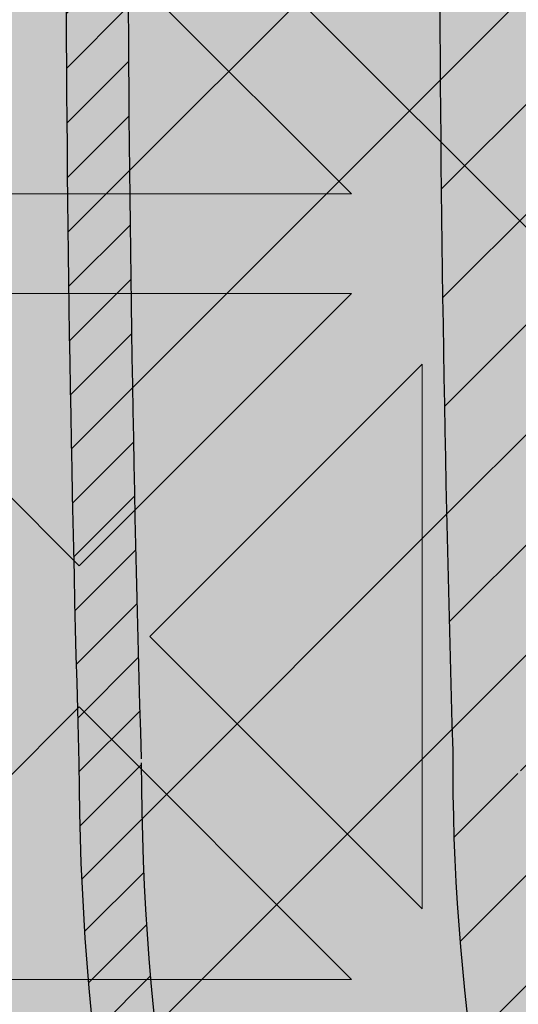
# Model space of a CAD drawing. Units: inches. Extents: x 844 to 2234, y 346 to 1084.
# Tile 11 of 93: x 1119.118 to 1120.394, y 691.183 to 693.702. Entities that reach past the tile are written whole.
import ezdxf

# ---------------------------------------------------------------- set-up
doc = ezdxf.new("R2010")
doc.units = ezdxf.units.IN
doc.header["$MEASUREMENT"] = 0
for name, color, linetype, lineweight in [('A-ANNO-DIMS', 2, 'Continuous', 18), ('furniture', 8, 'Continuous', 18), ('RA-AP-01$0$INT', 35, 'Continuous', 5)]:
    doc.layers.add(name, color=color, linetype=linetype, lineweight=lineweight)
doc.layers.add('RA-AP-01$0$FURN', color=3, linetype='Continuous')
doc.layers.add('RA-AP-01$0$WOOD', color=64, linetype='Continuous')
doc.styles.get("Standard").update_dxf_attribs({"font": 'arial.ttf'})
doc.dimstyles.get("Standard").update_dxf_attribs({"dimtxt": 6, "dimasz": 3, "dimexe": 0.18, "dimexo": 0.0625, "dimgap": 0.09, "dimtad": 0, "dimtih": 1, "dimtoh": 1, "dimdec": 1, "dimzin": 0, "dimdsep": 46, "dimlunit": 3, "dimtxsty": 'Standard', "dimblk": 'ARCHTICK', "dimcen": 0.09, "dimadec": 0, "dimazin": 0, "dimtfac": 1, "dimtdec": 1, "dimtofl": 0, "dimtmove": 0, "dimatfit": 3, "dimfxl": 1, "dimtolj": 1, "dimtzin": 0, "dimarcsym": 0})

# ---------------------------------------------------------------- blocks, each defined once
blk = doc.blocks.new('A$C18D01794')
at = {"layer": 'RA-AP-01$0$INT'}
h = blk.add_hatch(color=256, dxfattribs=at)
h.paths.add_polyline_path([(4.585917135068449, -6.356712009588271), (4.555206456959269, -6.35671200958746), (4.555206456959137, -6.387422687716308), (4.874495778835233, -6.706712009592356), (4.90520645695423, -6.676001331474049)])
h.paths.add_polyline_path([(5.255206456948813, -6.387422687716306), (5.255206456948682, -6.356712009605972), (5.224495778822613, -6.356712009605161), (4.905206456953498, -6.676001331474273), (4.935917135072151, -6.706712009592924)])
h.paths.add_polyline_path([(4.935917135072559, -6.706712009592068), (4.905206456953564, -6.737422687710376), (5.255206456951813, -7.087422687708613), (5.255206456951549, -7.026001331471008)])
h.paths.add_polyline_path([(4.555206456956399, -7.026001331471013), (4.555206456956134, -7.087422687708616), (4.905206456953821, -6.737422687710943), (4.874495778835166, -6.70671200959229)])
h = blk.add_hatch(color=256, dxfattribs=at)
h.paths.add_polyline_path([(4.585917135068448, -6.356712009588273), (4.614201406330596, -6.356712009589021), (4.668846067270487, -6.411356670531338), (4.723490728212344, -6.356712009591912), (4.771774999457151, -6.35671200959319), (4.826419660396886, -6.411356670535356), (4.862780050090322, -6.374996280843536), (4.844495778842715, -6.356712009595112), (4.862780050090411, -6.356712009595595), (4.905206456960182, -6.399138416468211), (4.947632863832445, -6.356712009597838), (4.965917135079675, -6.356712009598322), (4.947632863831759, -6.374996280845421), (4.983993253523576, -6.411356670538857), (5.038637914464627, -6.356712009600247), (5.08692218571208, -6.356712009601523), (5.141566846649976, -6.411356670541852), (5.196211507589851, -6.356712009604411), (5.224495778822615, -6.356712009605161), (4.905206456953975, -6.676001331473793)])
h.paths.add_polyline_path([(4.895206456956031, -6.637717060225675), (4.895206456958921, -6.528427738347902), (4.840561796018589, -6.583072399285802)], flags=16)
h.paths.add_polyline_path([(4.915206456955638, -6.637717060226121), (4.969851117895509, -6.583072399288678), (4.915206456957609, -6.528427738348344)], flags=16)
h.paths.add_polyline_path([(4.826419660395175, -6.568930263661755), (4.881064321335613, -6.514285602723745), (4.771774999456703, -6.514285602720857)], flags=16)
h.paths.add_polyline_path([(4.983993253519558, -6.568930263665262), (5.038637914460456, -6.514285602726792), (4.929348592581548, -6.514285602724816)], flags=16)
h.paths.add_polyline_path([(4.881064321336025, -6.494285602723742), (4.826419660397532, -6.439640941782821), (4.771774999457062, -6.494285602720859)], flags=16)
h.paths.add_polyline_path([(4.929348592582019, -6.494285602724817), (5.038637914460982, -6.494285602726792), (4.983993253522945, -6.439640941786327)], flags=16)
h.paths.add_polyline_path([(4.895206456960191, -6.480143467100443), (4.895206456962115, -6.407422687715913), (4.876922185715016, -6.389138416467584), (4.840561796021581, -6.425498806159401)], flags=16)
h.paths.add_polyline_path([(4.915206456958487, -6.480143467100889), (4.969851117899527, -6.425498806162279), (4.933490728206909, -6.389138416468043), (4.9152064569598, -6.40742268771434)], flags=16)
h.paths.add_polyline_path([(4.757632863832376, -6.480143467096812), (4.812277524772842, -6.425498806158772), (4.757632863834348, -6.370854145217844)], flags=16)
h.paths.add_polyline_path([(4.737632863832376, -6.480143467096286), (4.737632863834348, -6.370854145217375), (4.682988202893906, -6.425498806155385)], flags=16)
h.paths.add_polyline_path([(5.05278005008503, -6.480143467103376), (5.052780050087917, -6.370854145224413), (4.998135389146995, -6.425498806162908)], flags=16)
h.paths.add_polyline_path([(5.072780050085024, -6.480143467103744), (5.127424711025931, -6.42549880616527), (5.072780050087916, -6.370854145224832)], flags=16)
h.paths.add_polyline_path([(4.935917135072783, -6.706712009592292), (5.255206456948811, -6.387422687716309), (5.255206456948932, -6.415706958964177), (5.200561796010279, -6.470351619902839), (5.255206456949403, -6.524996280841948), (5.25520645694961, -6.5732805520894), (5.200561796009787, -6.627925213029239), (5.236922185702417, -6.664285602721864), (5.255206456949919, -6.646001331474357), (5.255206456949998, -6.664285602721898), (5.212780050078687, -6.706712009592262), (5.25520645695036, -6.749138416463932), (5.255206456950438, -6.767422687711313), (5.236922185702424, -6.749138416463297), (5.200561796009796, -6.785498806155928), (5.255206456950753, -6.840143467096874), (5.25520645695096, -6.888427738341682), (5.200561796010322, -6.943072399282328), (5.255206456951428, -6.997717060223427), (5.255206456951547, -7.026001331471006)])
h.paths.add_polyline_path([(5.042988202883395, -6.785498806155427), (5.097632863823085, -6.840143467095101), (5.097632863822622, -6.730854145216193)], flags=16)
h.paths.add_polyline_path([(5.028846067259663, -6.771356670531693), (5.083490728198774, -6.716712009592573), (4.974201406321001, -6.716712009593042)], flags=16)
h.paths.add_polyline_path([(5.117632863823087, -6.840143467095186), (5.172277524762331, -6.785498806155926), (5.11763286382262, -6.730854145216225)], flags=16)
h.paths.add_polyline_path([(5.08349072819877, -6.696712009593886), (5.028846067259652, -6.642067348654775), (4.974201406320998, -6.696712009593438)], flags=16)
h.paths.add_polyline_path([(5.131774999446817, -6.854285602718917), (5.186419660386065, -6.799640941779662), (5.241064321325782, -6.854285602719365)], flags=17)
h.paths.add_polyline_path([(5.131774999446228, -6.716712009592374), (5.186419660386065, -6.771356670532194), (5.222780050079488, -6.734996280838764), (5.204495778832781, -6.716712009592063)], flags=16)
h.paths.add_polyline_path([(5.097632863822613, -6.682569873970264), (5.097632863823061, -6.573280552091354), (5.042988202883383, -6.627925213031044)], flags=16)
h.paths.add_polyline_path([(5.131774999446899, -6.874285602718915), (5.241064321325809, -6.874285602719364), (5.186419660386591, -6.928930263658598)], flags=17)
h.paths.add_polyline_path([(5.131774999446226, -6.696712009594078), (5.204495778830767, -6.696712009594374), (5.22278005007868, -6.67842773834687), (5.186419660386049, -6.642067348654249)], flags=16)
h.paths.add_polyline_path([(5.11763286382262, -6.682569873970225), (5.17227752476232, -6.627925213030515), (5.117632863823064, -6.573280552091267)], flags=16)
h.paths.add_polyline_path([(5.186419660386069, -6.613783077405491), (5.241064321325754, -6.559138416465795), (5.131774999446791, -6.559138416466263)], flags=16)
h.paths.add_polyline_path([(5.131774999446872, -6.539138416466263), (5.24106432132578, -6.539138416465794), (5.186419660386554, -6.484493755526573)], flags=16)
h.paths.add_polyline_path([(5.255206456951811, -7.08742268770861), (5.255206456951895, -7.106712009588038), (4.555206456956052, -7.106712009588038), (4.555206456956136, -7.087422687708617), (4.905206456953973, -6.737422687710788)])
h.paths.add_polyline_path([(4.983993253513404, -6.8444937555241), (4.92934859257295, -6.899138416462108), (5.03863791445186, -6.899138416465014)], flags=16)
h.paths.add_polyline_path([(4.969851117889988, -6.83035161990006), (4.915206456952556, -6.775706958960171), (4.915206456949648, -6.884996280837944)], flags=16)
h.paths.add_polyline_path([(4.929348592572535, -6.919138416462105), (4.983993253511019, -6.973783077403037), (5.038637914451496, -6.919138416465012)], flags=16)
h.paths.add_polyline_path([(5.052780050074912, -6.93328055208906), (4.998135389134438, -6.987925213027088), (5.052780050072919, -7.042569873968025)], flags=16)
h.paths.add_polyline_path([(5.07278005007491, -6.933280552089588), (5.072780050072918, -7.042569873968497), (5.127424711013374, -6.987925213030498)], flags=16)
h.paths.add_polyline_path([(4.89520645695295, -6.775706958959721), (4.840561796013067, -6.830351619897157), (4.895206456950961, -6.884996280837494)], flags=16)
h.paths.add_polyline_path([(4.915206456948365, -6.933280552085403), (4.915206456946434, -7.006001331471951), (4.933490728192729, -7.024285602719066), (4.969851117886972, -6.987925213026453)], flags=16)
h.paths.add_polyline_path([(4.881064321327021, -6.899138416461022), (4.82641966038902, -6.84449375552057), (4.771774999448108, -6.899138416459029)], flags=16)
h.paths.add_polyline_path([(4.895206456950073, -6.933280552084951), (4.840561796009022, -6.987925213023558), (4.876922185700835, -7.024285602716997), (4.895206456948749, -7.006001331469487)], flags=16)
h.paths.add_polyline_path([(4.983993253510392, -7.0020673486505), (4.947632863816944, -7.038427738342319), (4.965917135064043, -7.05671200959023), (5.038637914448995, -7.056712009591555)], flags=16)
h.paths.add_polyline_path([(4.881064321326543, -6.91913841646102), (4.771774999447578, -6.919138416459031), (4.826419660385607, -6.973783077399508)], flags=16)
h.paths.add_polyline_path([(4.905206456946447, -7.014285602717636), (4.862780050074785, -7.056712009588352), (4.947632863816685, -7.056712009589775)], flags=16)
h.paths.add_polyline_path([(5.14156684663679, -7.002067348654549), (5.086922185696452, -7.056712009592438), (5.196211507574223, -7.056712009594425)], flags=16)
h.paths.add_polyline_path([(4.8264196603837, -7.002067348646972), (4.771774999442643, -7.056712009585575), (4.8444957788276, -7.056712009587508), (4.862780050075511, -7.038427738340416)], flags=16)
h.paths.add_polyline_path([(4.812277524760289, -6.98792521302292), (4.757632863822258, -6.933280552082447), (4.757632863819352, -7.042569873961408)], flags=16)
h.paths.add_polyline_path([(4.73763286382226, -6.933280552082079), (4.682988202881349, -6.987925213020536), (4.737632863819352, -7.04256987396099)], flags=16)
h.paths.add_polyline_path([(4.723490728195188, -7.056712009584289), (4.668846067257299, -7.002067348643949), (4.614201406317417, -7.056712009581383)], flags=16)
h.paths.add_polyline_path([(4.597632863829262, -6.706712009592262), (4.555206456957951, -6.664285602721896), (4.555206456958029, -6.646001331474357), (4.573490728205535, -6.664285602721864), (4.609851117898167, -6.627925213029238), (4.555206456958338, -6.573280552089402), (4.555206456958546, -6.524996280841952), (4.60985111789767, -6.470351619902839), (4.555206456959015, -6.415706958964177), (4.555206456959138, -6.387422687716309), (4.874495778835167, -6.70671200959229), (4.5552064569564, -7.026001331471015), (4.555206456956523, -6.997717060223433), (4.609851117897629, -6.94307239928233), (4.555206456956988, -6.888427738341681), (4.555206456957198, -6.840143467096881), (4.609851117898153, -6.78549880615593), (4.573490728205528, -6.749138416463297), (4.555206456957507, -6.76742268771132), (4.555206456957585, -6.749138416463933)])
h.paths.add_polyline_path([(4.712780050085332, -6.730854145216195), (4.712780050084863, -6.840143467095105), (4.767424711024555, -6.785498806155427)], flags=16)
h.paths.add_polyline_path([(4.726922185709173, -6.716712009592573), (4.781566846648288, -6.771356670531693), (4.836211507586949, -6.716712009593043)], flags=16)
h.paths.add_polyline_path([(4.692780050085327, -6.730854145216225), (4.638135389145619, -6.785498806155928), (4.692780050084865, -6.840143467095185)], flags=16)
h.paths.add_polyline_path([(4.726922185709182, -6.696712009593886), (4.836211507586949, -6.696712009593436), (4.7815668466483, -6.642067348654773)], flags=16)
h.paths.add_polyline_path([(4.678637914461726, -6.71671200959237), (4.605917135075169, -6.716712009592063), (4.587632863828464, -6.734996280838766), (4.623993253521887, -6.771356670532195)], flags=16)
h.paths.add_polyline_path([(4.712780050085336, -6.68256987397026), (4.767424711024568, -6.627925213031042), (4.71278005008489, -6.573280552091352)], flags=16)
h.paths.add_polyline_path([(4.678637914461726, -6.696712009594076), (4.623993253521899, -6.642067348654247), (4.587632863829271, -6.67842773834687), (4.605917135077185, -6.696712009594376)], flags=16)
h.paths.add_polyline_path([(4.692780050085336, -6.682569873970228), (4.692780050084889, -6.573280552091267), (4.638135389145632, -6.627925213030515)], flags=16)
h.paths.add_polyline_path([(4.623993253521885, -6.799640941779662), (4.678637914461131, -6.854285602718915), (4.56934859258217, -6.854285602719365)], flags=17)
h.paths.add_polyline_path([(4.623993253521901, -6.613783077405509), (4.678637914461158, -6.559138416466263), (4.569348592582195, -6.559138416465795)], flags=16)
h.paths.add_polyline_path([(4.678637914461051, -6.874285602718915), (4.623993253521361, -6.928930263658598), (4.569348592582143, -6.874285602719364)], flags=17)
h.paths.add_polyline_path([(4.678637914461076, -6.539138416466263), (4.623993253521399, -6.484493755526573), (4.569348592582167, -6.539138416465796)], flags=16)
h = blk.add_hatch(color=256, dxfattribs=at)
h.paths.add_polyline_path([(4.781566846647504, -6.771356670530272), (4.836211507586161, -6.716712009591613), (4.726922185708388, -6.716712009591159)])
h.paths.add_polyline_path([(4.836211507586161, -6.696712009592008), (4.781566846647504, -6.642067348653354), (4.726922185708388, -6.69671200959247)])
h.paths.add_polyline_path([(4.76742471102377, -6.627925213029623), (4.712780050084083, -6.57328055208994), (4.712780050084542, -6.68256987396885)])
h.paths.add_polyline_path([(4.692780050084544, -6.682569873968819), (4.692780050084084, -6.573280552089856), (4.638135389144834, -6.627925213029111)])
h.paths.add_polyline_path([(4.678637914460932, -6.696712009592669), (4.623993253521102, -6.642067348652844), (4.587632863827676, -6.678427738346266), (4.605917135074382, -6.696712009592973)])
h.paths.add_polyline_path([(4.573490728204743, -6.664285602721736), (4.60985111789737, -6.627925213029108), (4.555206456957541, -6.573280552089279), (4.555206456957237, -6.646001331474231)])
h.paths.add_polyline_path([(4.623993253521098, -6.613783077405377), (4.67863791446035, -6.559138416466126), (4.56934859258139, -6.559138416465669)])
h.paths.add_polyline_path([(4.678637914460275, -6.539138416466126), (4.623993253520583, -6.48449375552644), (4.56934859258136, -6.539138416465672)])
h.paths.add_polyline_path([(4.609851117896854, -6.470351619902707), (4.555206456958196, -6.415706958964051), (4.555206456957738, -6.524996280841822)])
h.paths.add_polyline_path([(4.597632863828475, -6.706712009592775), (4.555206456957283, -6.664285602721582), (4.555206456956805, -6.749138416463489)])
h.paths.add_polyline_path([(4.678637914460932, -6.716712009590963), (4.605917135076396, -6.71671200959066), (4.587632863828479, -6.734996280838164), (4.623993253521104, -6.771356670530792)])
h.paths.add_polyline_path([(4.692780050084091, -6.840143467093776), (4.692780050084548, -6.730854145214809), (4.638135389144834, -6.785498806154524)])
h.paths.add_polyline_path([(4.767424711023772, -6.785498806154004), (4.712780050084545, -6.730854145214786), (4.712780050084089, -6.840143467093692)])
h.paths.add_polyline_path([(4.67863791446036, -6.854285602718778), (4.623993253521105, -6.799640941779527), (4.569348592581399, -6.854285602719237)])
h.paths.add_polyline_path([(4.609851117897371, -6.785498806155798), (4.573490728204743, -6.74913841646317), (4.555206456957237, -6.767422687710675), (4.555206456957548, -6.840143467095629)])
h.paths.add_polyline_path([(4.623993253520596, -6.928930263658465), (4.67863791446028, -6.874285602718778), (4.569348592581367, -6.874285602719238)])
h.paths.add_polyline_path([(4.609851117896867, -6.943072399282199), (4.555206456957749, -6.888427738343082), (4.55520645695821, -6.997717060220857)])
for p, q in [((4.874495778835167, -6.70671200959229), (4.555206456956399, -7.026001331471013)), ((4.60591713507677, -6.716712009592063), (4.678637914461721, -6.716712009592372)), ((4.678637914461721, -6.716712009592372), (4.623993253521887, -6.771356670532195)), ((4.692780050085331, -6.730854145216223), (4.638135389145619, -6.785498806155928)), ((4.692780050084865, -6.840143467095186), (4.692780050085331, -6.730854145216223)), ((4.623993253521889, -6.771356670532195), (4.587632863829264, -6.734996280839565)), ((4.692780050084865, -6.840143467095186), (4.638135389145619, -6.785498806155928)), ((4.56934859258217, -6.854285602719365), (4.623993253521885, -6.799640941779662)), ((4.678637914461133, -6.854285602718915), (4.623993253521885, -6.799640941779662)), ((4.678637914461133, -6.854285602718915), (4.56934859258217, -6.854285602719365)), ((4.678637914461051, -6.874285602718915), (4.569348592582142, -6.874285602719364)), ((4.623993253521363, -6.928930263658596), (4.678637914461051, -6.874285602718915))]:
    blk.add_line(p, q, dxfattribs=at)
blk = doc.blocks.new('A$C32926AE1')
at = {"layer": 'RA-AP-01$0$FURN'}
h = blk.add_hatch(dxfattribs=at)
h.set_pattern_fill('ANSI31', color=256, scale=0.1, style=0)
h.set_pattern_definition([(45, (0, 0), (-0.0088388347648318, 0.0088388347648318), [])])
edge = h.paths.add_edge_path(flags=16)
edge.add_arc((4.904771284329206, 4.246793130718756), 0.2603971832811541, 75.22398030683196, 104.7760196931204)
edge.add_arc((4.904771284329206, 4.246793130718756), 0.2603971832811541, 75.223980306832, 104.77601969312039, ccw=False)
edge = h.paths.add_edge_path(flags=16)
edge.add_arc((4.904771284329206, 4.067062675376612), 0.2603971832811541, 255.2239803068796, 284.776019693168)
edge.add_arc((4.904771284329206, 4.067062675376612), 0.2603971832811541, 255.22398030687958, 284.77601969316805, ccw=False)
edge = h.paths.add_edge_path(flags=0)
edge.add_arc((4.904771284329206, 4.067062675376612), 0.2603971832811541, 255.2239803068796, 284.776019693168)
edge.add_arc((4.904771284329206, 4.067062675376612), 0.2603971832811541, 255.22398030687958, 284.77601969316805, ccw=False)
edge = h.paths.add_edge_path(flags=0)
edge.add_arc((4.904771284329206, 4.067062675376612), 0.2603971832811541, 255.2239803068796, 284.776019693168)
edge.add_arc((4.904771284329206, 4.067062675376612), 0.2603971832811541, 255.22398030687958, 284.77601969316805, ccw=False)
edge = h.paths.add_edge_path()
edge.add_arc((4.604388392048174, 4.588829985554312), 0.1599999999999918, 342.3781640246255, 354.4317409793762)
edge.add_arc((5.090145208887507, 4.43216705527679), 0.3503971832811637, 162.0091218307731, 180.3186872093483)
edge.add_arc((5.205154176610243, 4.588829985554953), 0.1599999999999917, 185.5682590208461, 197.6218359767349)
edge.add_arc((4.904771284329229, 4.246793130718735), 0.3503971832811761, 72.00912183053516, 107.9908781690354)
edge.add_arc((9.535952835716557, 4.28682295566602), 4.798342501046485, 178.2875002453811, 181.5576802719453)
edge.add_arc((4.719397359771122, 4.43216705527679), 0.3503971832811637, 359.6813127906516, 377.9908781692269)
edge.add_arc((9.535967292294904, 4.286822350292874), 4.778371420254705, 178.2965938931842, 181.5667745797229)
edge.add_arc((4.719397359771122, 4.43216705527679), 0.3303971832811637, 359.6813127906516, 377.9908781692269)
edge.add_arc((0.2735752763637294, 4.286822350292874), 4.7783714202547, 358.4332254202771, 361.7034061068158)
edge.add_arc((5.061434214606998, 4.732549947558029), 0.1600000000000254, 252.3781640250584, 264.4317409792362)
edge.add_arc((4.748108354051257, 4.732549947558012), 0.1600000000000541, 275.5682590208426, 287.6218359759532)
edge.add_arc((4.604388392048115, 4.588829985554317), 0.1800000000000505, 342.3567572500182, 349.3735009646207)
edge.add_arc((5.205154176610254, 4.588829985554976), 0.1800000000000069, 190.6264990356027, 197.6432427513933)
edge.add_arc((5.061434214607106, 4.732549947558013), 0.1800000000000424, 252.3567572496606, 259.3735009644582)
edge.add_arc((4.904771284329208, 4.246793130718737), 0.3303971832811676, 71.99844483668534, 108.0015551637021)
edge.add_arc((4.748108354051414, 4.732549947558045), 0.1800000000000547, 280.6264990355479, 287.6432427495938)
edge.add_arc((5.090145208887514, 4.432167055276789), 0.2803971832811691, 162.8706300666893, 180.816523289902)
edge.add_arc((4.719397359771136, 4.432167055276689), 0.2803971832811534, 359.183476710103, 377.1293699333214)
edge.add_arc((4.904771284329222, 4.246793130718737), 0.2803971832811769, 72.87063006672916, 107.1293699332334)
edge.add_arc((5.090145208887522, 4.432167055276788), 0.2603971832811776, 165.2239803068007, 180.9953123810312)
edge.add_arc((4.719397359771141, 4.432167055276699), 0.2603971832811458, 359.0046876189768, 374.7760196932087)
edge.add_arc((5.090145208887507, 4.43216705527679), 0.3303971832811637, 162.0091218307731, 180.3186872093483)
edge.add_arc((9.53595427642584, 4.285015535491528), 4.728345371032053, 178.265043920078, 181.5679956281801)
edge.add_arc((0.2735882922327999, 4.285015535491582), 4.728345371032045, 358.4320043718193, 361.7349560799204)
edge.add_arc((9.535953591267507, 4.284458026472751), 4.708343996644348, 178.2573054306777, 181.5704995759608)
edge.add_arc((0.273588977391114, 4.284458026472785), 4.708343996644358, 358.4295004240388, 361.7426945693213)
edge.add_arc((0.2735889773911131, 4.029397779622582), 4.708343996644359, 358.2573054306787, 361.5704995759613)
edge.add_arc((9.535953591267518, 4.029397779622618), 4.708343996644359, 178.4295004240391, 181.7426945693223)
edge.add_arc((0.2735882922327901, 4.028840270603786), 4.728345371032054, 358.2650439200796, 361.5679956281808)
edge.add_arc((9.53595427642584, 4.028840270603841), 4.728345371032054, 178.4320043718199, 181.7349560799219)
edge.add_arc((0.2735752763637302, 4.027033455802493), 4.778371420254699, 358.2965938931842, 361.5667745797229)
edge.add_arc((4.719397359771122, 3.881688750818578), 0.3303971832811637, 342.0091218307731, 360.3186872093484)
edge.add_arc((5.090145208887507, 3.881688750818578), 0.3303971832811637, 179.6813127906516, 197.9908781692269)
edge.add_arc((9.535967292294904, 4.027033455802493), 4.778371420254705, 178.433225420277, 181.7034061068158)
edge.add_arc((4.719397359771122, 3.881688750818578), 0.3503971832811637, 342.0091218307731, 360.3186872093484)
edge.add_arc((9.53595283571655, 4.027032850429349), 4.79834250104648, 178.4423197280546, 181.7124997546188)
edge.add_arc((4.719397359771141, 3.881688750818669), 0.2603971832811458, 345.2239803067913, 360.9953123810232)
edge.add_arc((5.090145208887522, 3.88168875081858), 0.2603971832811776, 179.0046876189687, 194.7760196931993)
edge.add_arc((4.904771284329222, 4.067062675376631), 0.2803971832811769, 252.8706300667665, 287.1293699332708)
edge.add_arc((4.719397359771136, 3.881688750818678), 0.2803971832811534, 342.8706300666787, 360.8165232898969)
edge.add_arc((5.090145208887514, 3.881688750818579), 0.2803971832811691, 179.183476710098, 197.1293699333106)
edge.add_arc((4.748108354051414, 3.581305858537323), 0.1800000000000547, 72.3567572504062, 79.37350096445199)
edge.add_arc((4.904771284329208, 4.067062675376631), 0.3303971832811676, 251.9984448362979, 288.0015551633146)
edge.add_arc((5.061434214607106, 3.581305858537355), 0.1800000000000424, 100.6264990355418, 107.6432427503394)
edge.add_arc((5.205154176610254, 3.725025820540392), 0.1800000000000069, 162.3567572486066, 169.3735009643972)
edge.add_arc((4.604388392048115, 3.725025820541051), 0.1800000000000505, 10.62649903537925, 17.64324274998182)
edge.add_arc((4.748108354051257, 3.581305858537356), 0.1600000000000541, 72.37816402404681, 84.43174097915735)
edge.add_arc((4.904771284329229, 4.067062675376632), 0.3503971832811761, 252.0091218309645, 287.9908781694648)
edge.add_arc((5.061434214606998, 3.581305858537339), 0.1600000000000254, 95.56825902076373, 107.6218359749416)
edge.add_arc((5.205154176610243, 3.725025820540414), 0.1599999999999917, 162.3781640232651, 174.4317409791539)
edge.add_arc((5.090145208887507, 3.881688750818578), 0.3503971832811637, 179.6813127906516, 197.9908781692269)
edge.add_arc((4.604388392048174, 3.725025820541056), 0.1599999999999918, 5.568259020623824, 17.62183597537444)
edge.add_arc((0.2735897329420762, 4.28682295566602), 4.798342501046482, 358.4423197280547, 361.7124997546188)
edge.add_arc((0.2735897329420691, 4.027032850429348), 4.798342501046489, 358.2875002453812, 361.5576802719453)
at = {"layer": 'RA-AP-01$0$WOOD'}
h = blk.add_hatch(color=256, dxfattribs=at)
h.dxf.hatch_style = 1
h.paths.add_polyline_path([(5.157430609644524, 4.573483066760929, -0.1009492694046607), (5.155401577623758, 4.593365984175333, -0.1842662638101597), (5.172249623284174, 4.638795604568598, 0.2056608120311276), (5.179560981299304, 4.661316324430096, 0.3614336704623542), (5.134352340494423, 4.706524965234944, 0.2056608120311297), (5.111831620632933, 4.699213607219793, -0.1842662638101113), (5.066402000239693, 4.682365561559342, -0.1055311479399994), (5.045656153913092, 4.68467289944697, 0.1567636581983829), (4.763886414745334, 4.684672899446966, -0.1055311479399895), (4.743140568418733, 4.68236556155934, -0.1842662638100833), (4.6977109480255, 4.69921360721979, 0.2056608120302612), (4.675190228164109, 4.706524965234949, 0.3614336704708441), (4.629981587358889, 4.66131632442871, 0.2056608120245944), (4.637292945374126, 4.638795604567974, -0.1842662638101024), (4.654140991034615, 4.59336598417475, -0.1009492694055169), (4.652111959013835, 4.573483066760181, 0.021410119221476), (4.629748025606143, 4.156712009541676, 0.0214101192214795), (4.652111959013809, 3.739940952323101, -0.1009492694059586), (4.654140991034615, 3.720058034908448, -0.1842662638100975), (4.637292945374126, 3.674628414515226, 0.2056608120245705), (4.629981587358889, 3.652107694654492, 0.3614336704708879), (4.675190228164113, 3.606899053848249, 0.2056608120302384), (4.697710948025501, 3.614210411863408, -0.1842662638100995), (4.743140568418738, 3.63105845752386, -0.1055311479402541), (4.763886414745388, 3.628751119636215, 0.1567636581983776), (5.045656153913137, 3.628751119636244, -0.1055311479397538), (5.066402000239692, 3.631058457523857, -0.1842662638101067), (5.111831620632931, 3.614210411863407, 0.2056608120310924), (5.134352340494417, 3.606899053848256, 0.3614336704624001), (5.179560981299307, 3.652107694653103, 0.2056608120311314), (5.172249623284175, 3.6746284145146, -0.1842662638101402), (5.155401577623758, 3.72005803490786, -0.1009492694051366), (5.15743060964455, 3.739940952322354, 0.0214101192215073), (5.179794543052287, 4.156712009541468, 0.0214101192215252)])
h.paths.add_polyline_path([(4.639748609479751, 4.156712009541513, 0.0213537860821624), (4.661970494867118, 3.741887061152232, -0.094075836301374), (4.664143710413708, 3.7196126951003, -0.1824818158568985), (4.644813765429836, 3.668037719127816, 0.2056608120245319), (4.639939526753007, 3.653023905887301, 0.3614336704710246), (4.676106439397173, 3.616856993242342, 0.2056608120302234), (4.691120252638095, 3.621731231919122, -0.1824818158602558), (4.742695228611606, 3.641061176902986, -0.1029891339458722), (4.766991894714349, 3.638256818950944, 0.156709409989566), (5.042550673941472, 3.638256818950105, -0.102989133958497), (5.066847340047078, 3.641061176902949, -0.1824818158594995), (5.118422316020358, 3.621731231919103, 0.2056608120311416), (5.133436129261316, 3.616856993242346, 0.3614336704621468), (5.169603041905217, 3.653023905886178, 0.2056608120310986), (5.164728803228477, 3.668037719127177, -0.1824818158565612), (5.145398858244737, 3.719612695099578, -0.0940758363009313), (5.147572073791232, 3.741887061151398, 0.0213537860822023), (5.169793959178681, 4.156712009541451, 0.0213537860822226), (5.147572073791203, 4.571536957931898, -0.0940758363005034), (5.145398858244737, 4.59381132398362, -0.1824818158565587), (5.164728803228476, 4.645386299956021, 0.2056608120311045), (5.169603041905216, 4.66040011319702, 0.3614336704621845), (5.133436129261313, 4.696567025840856, 0.2056608120310773), (5.118422316020359, 4.691692787164098, -0.182481815859508), (5.066847340047078, 4.67236284218025, -0.1029891339584606), (5.04255067394148, 4.675167200133092, 0.156709409989566), (4.766991894714357, 4.675167200132257, -0.1029891339458842), (4.742695228611611, 4.672362842180213, -0.1824818158602725), (4.691120252638095, 4.691692787164077, 0.2056608120302152), (4.676106439397174, 4.696567025840858, 0.3614336704710363), (4.639939526753005, 4.660400113195899, 0.2056608120245495), (4.644813765429837, 4.645386299955384, -0.1824818158568934), (4.664143710413708, 4.593811323982902, -0.0940758363009187), (4.661970494867149, 4.571536957931074, 0.021353786082177)], flags=16)
h.paths.add_polyline_path([(5.129794543052235, 4.432167055276933, -0.0141661062790638), (5.130152669293814, 4.156927903047693, -0.0141661062790647), (5.129794543052234, 3.881688750818433, -0.0785247771143638), (5.10979738006795, 3.755143611847103, 0.0945969212073497), (5.105408519571111, 3.717898134952927, 0.1043170707844957), (5.116074640131521, 3.670385395016088, 0.1043170707864965), (5.068561900193738, 3.681051515576561, 0.09459692119553), (5.031316423304057, 3.676662655080835, -0.1580239521427272), (4.778226145355827, 3.676662655080367, 0.0945969211986668), (4.740980668464973, 3.681051515576592, 0.1043170707882822), (4.693467928526415, 3.670385395015844, 0.1043170707867916), (4.704134049087309, 3.717898134953662, 0.0945969211972894), (4.69974518859162, 3.755143611844042, -0.0785247771163196), (4.679748025606343, 3.881688750818406, -0.0141661062790663), (4.679389899364763, 4.156927903047693, -0.0141661062790672), (4.679748025606343, 4.432167055276998, -0.0785247771163064), (4.699745188591625, 4.55871219425134, 0.094596921197333), (4.704134049087308, 4.595957671141738, 0.1043170707867205), (4.693467928526416, 4.643470411079523, 0.1043170707882628), (4.740980668464965, 4.632804290518776, 0.0945969211988114), (4.778226145355874, 4.637193151015016, -0.158023952142669), (5.031316423304015, 4.637193151014546, 0.0945969211956361), (5.068561900193736, 4.632804290518806, 0.1043170707864979), (5.11607464013152, 4.643470411079278, 0.1043170707844617), (5.105408519571112, 4.595957671142455, 0.0945969212074597), (5.109797380067959, 4.558712194248236, -0.0785247771143467)], flags=0)
h.paths.add_polyline_path([(5.119794532311105, 4.432259799204851, -0.0142000800617244), (5.120156169157484, 4.156927903047701, -0.0142000800617277), (5.119794532311105, 3.881596006890482, -0.0784894509520253), (5.100273383573699, 3.758192358677797, 0.0940138827242913), (5.095413455884425, 3.717477693979438, 0.0606271852308753), (5.099615656341024, 3.686844378806616, 0.0606271852322524), (5.068982341167493, 3.691046579263239, 0.0940138827010453), (5.028267676478798, 3.686186651576848, -0.1580706864508061), (4.781274892180912, 3.686186651576435, 0.0940138827026903), (4.740560227491556, 3.691046579263279, 0.0606271852339895), (4.709926912317155, 3.686844378806508, 0.0606271852329405), (4.714129112773991, 3.717477693980356, 0.094013882701304), (4.709269185087677, 3.758192358669163, -0.0784894509577193), (4.689748036347473, 3.881596006890469, -0.014200080061729), (4.689386399501094, 4.156927903047709, -0.0142000800617217), (4.689748036347473, 4.432259799204808, -0.078489450957724), (4.709269185087651, 4.555663447426125, 0.0940138827014585), (4.714129112773992, 4.596378112114996, 0.0606271852329731), (4.709926912317154, 4.62701142728886, 0.0606271852340196), (4.74056022749157, 4.622809226832087, 0.0940138827024997), (4.781274892180847, 4.627669154518912, -0.1580706864508359), (5.028267676478777, 4.627669154518526, 0.0940138827010946), (5.068982341167492, 4.622809226832129, 0.060627185232254), (5.099615656341024, 4.627011427288751, 0.0606271852308727), (5.095413455884425, 4.59637811211593, 0.0940138827241088), (5.100273383573675, 4.555663447417647, -0.0784894509520978)], flags=0)
h.paths.add_polyline_path([(5.06978912287499, 4.430218106756144, -0.014241683694547), (5.070173729147532, 4.156927903047672, -0.0142416836945458), (5.06978912287499, 3.883637699339223, -0.0800609523125196), (5.052662118612511, 3.773463122773442, 0.0526421978001116), (5.04590916754064, 3.740550867606997, 0.0526421977992423), (5.012996912374707, 3.73379791653534, -0.1583028414718258), (4.796545656286308, 3.73379791653451, 0.0526421978034211), (4.763633401117837, 3.740550867607021, 0.0526421978018622), (4.756880450045755, 3.773463122774558, -0.0800609523117106), (4.739753445783639, 3.883637699339268, -0.0142416836945435), (4.739368839511098, 4.156927903047671, -0.0142416836945477), (4.739753445783639, 4.430218106756155, -0.0800609523116345), (4.75688045004574, 4.540392683320762, 0.052642197801941), (4.763633401117837, 4.573304938488346, 0.0526421978035071), (4.796545656286361, 4.580057889560873, -0.1583028414717561), (5.012996912374669, 4.580057889560039, 0.0526421977993048), (5.04590916754064, 4.57330493848837, 0.0526421978002057), (5.052662118612529, 4.540392683321868, -0.080060952312477)], flags=0)
h.paths.add_polyline_path([(5.049789715110557, 4.43038092723357, -0.0143097550741839), (5.05018085590259, 4.156927903047715, -0.0143097550741854), (5.049789715110558, 3.883474878861827, -0.0800685599149176), (5.03362098255317, 3.779581877367999, 0.0306258898956367), (5.028241146483733, 3.758218888663947, 0.0306258898977031), (5.006878157778253, 3.75283905259408, -0.1583983521624096), (4.802664410878162, 3.752839052594731, 0.0306258898946014), (4.781301422174808, 3.758218888663924, 0.0306258898967912), (4.775921586105202, 3.779581877368794, -0.080068559914251), (4.759752853548071, 3.883474878861786, -0.0143097550741854), (4.759361712756037, 4.156927903047671, -0.0143097550741854), (4.759752853548071, 4.430380927233557, -0.0800685599142479), (4.775921586105193, 4.534273928726546, 0.0306258898968306), (4.781301422174808, 4.555636917431444, 0.0306258898945754), (4.802664410878143, 4.561016753500631, -0.1583983521624168), (5.006878157778244, 4.561016753501291, 0.0306258898977177), (5.028241146483733, 4.555636917431421, 0.0306258898958182), (5.03362098255321, 4.534273928727244, -0.080068559914796)], flags=0)
h.paths.add_polyline_path([(4.999766070382627, 4.428171244713864, -0.0143443147609634), (5.000198441819402, 4.156927903047689, -0.0143443147609612), (4.999766070382627, 3.885684561381556, -0.0784641635803329), (4.987356730658798, 3.799103304488872, -0.1506053783831347), (4.822185837999821, 3.79910330448882, -0.0784641635803318), (4.809776498276007, 3.885684561381509, -0.014344314760963), (4.809344126839227, 4.156927903047677, -0.0143443147609645), (4.809776498276007, 4.428171244713873, -0.0784641635803192), (4.822185837999822, 4.514752501606549, -0.1506053783831338), (4.987356730658798, 4.514752501606494, -0.078464163580285)], flags=0)
h.paths.add_polyline_path([(4.979755254238824, 4.42764379880488, -0.0143772539198268), (4.980205517789977, 4.156927903047693, -0.0143772539198275), (4.979755254238824, 3.886212007290489, -0.0689242507424422), (4.971183264704897, 3.815276770442801, -0.1296645318904179), (4.838359303953726, 3.815276770442746, -0.0689242507424186), (4.829787314419809, 3.886212007290419, -0.0143772539198292), (4.829337050868653, 4.156927903047653, -0.0143772539198325), (4.829787314419809, 4.427643798804946, -0.0689242507424211), (4.838359303953725, 4.498579035652621, -0.1296645318904187), (4.971183264704897, 4.498579035652565, -0.0689242507424401)], flags=0)
h = blk.add_hatch(color=256, dxfattribs=at)
h.dxf.hatch_style = 1
h.paths.add_polyline_path([(5.145398858244737, 4.59381132398362, -0.1824818158565616), (5.164728803228476, 4.645386299956021, 0.2056608120311045), (5.169603041905216, 4.66040011319702, 0.3614336704621845), (5.133436129261313, 4.696567025840856, 0.2056608120310773), (5.118422316020359, 4.691692787164098, -0.182481815859508), (5.066847340047078, 4.67236284218025, -0.1029891339584606), (5.04255067394148, 4.675167200133092, 0.156709409989566), (4.766991894714357, 4.675167200132257, -0.1029891339458842), (4.742695228611611, 4.672362842180213, -0.1824818158602725), (4.691120252638095, 4.691692787164077, 0.2056608120302152), (4.676106439397174, 4.696567025840858, 0.3614336704710363), (4.639939526753005, 4.660400113195899, 0.2056608120245495), (4.644813765429837, 4.645386299955384, -0.1824818158568934), (4.664143710413708, 4.593811323982902, -0.0940758363009187), (4.661970494867149, 4.571536957931074, 0.0213537860821772), (4.639748609479751, 4.156712009541507, 0.0213537860821625), (4.661970494867119, 3.741887061152226, -0.0940758363013071), (4.664143710413708, 3.719612695100309, -0.1824818158569294), (4.644813765429836, 3.668037719127816, 0.2056608120245319), (4.639939526753007, 3.653023905887301, 0.3614336704710246), (4.676106439397173, 3.616856993242342, 0.2056608120302234), (4.691120252638095, 3.621731231919122, -0.1824818158602558), (4.742695228611606, 3.641061176902986, -0.1029891339458722), (4.766991894714349, 3.638256818950944, 0.156709409989566), (5.042550673941472, 3.638256818950105, -0.102989133958497), (5.066847340047078, 3.641061176902949, -0.1824818158594995), (5.118422316020358, 3.621731231919103, 0.2056608120311416), (5.133436129261316, 3.616856993242346, 0.3614336704621468), (5.169603041905217, 3.653023905886178, 0.2056608120310986), (5.164728803228477, 3.668037719127177, -0.1824818158565612), (5.145398858244737, 3.719612695099578, -0.0940758363009313), (5.147572073791232, 3.741887061151398, 0.0213537860822023), (5.169793959178681, 4.156712009541451, 0.0213537860822226), (5.147572073791203, 4.571536957931898, -0.0940758363004996)])
h.paths.add_polyline_path([(5.109797380067958, 4.55871219424824, -0.0785247771143472), (5.129794543052234, 4.432167055276936, -0.0141661062790644), (5.130152669293814, 4.156927903047685, -0.014166106279066), (5.129794543052234, 3.881688750818401, -0.0785247771143517), (5.109797380067946, 3.755143611847092, 0.0945969212073132), (5.105408519571111, 3.717898134952929, 0.1043170707844995), (5.116074640131521, 3.670385395016088, 0.1043170707864965), (5.068561900193738, 3.681051515576561, 0.09459692119553), (5.031316423304057, 3.676662655080835, -0.1580239521427272), (4.778226145355827, 3.676662655080367, 0.0945969211986668), (4.740980668464973, 3.681051515576592, 0.1043170707882822), (4.693467928526415, 3.670385395015844, 0.1043170707867916), (4.704134049087309, 3.717898134953662, 0.0945969211972894), (4.69974518859162, 3.755143611844042, -0.0785247771163196), (4.679748025606343, 3.881688750818406, -0.0141661062790663), (4.679389899364763, 4.156927903047693, -0.0141661062790672), (4.679748025606343, 4.432167055276998, -0.0785247771163064), (4.699745188591625, 4.55871219425134, 0.094596921197333), (4.704134049087308, 4.595957671141738, 0.1043170707867205), (4.693467928526416, 4.643470411079523, 0.1043170707882628), (4.740980668464965, 4.632804290518776, 0.0945969211988114), (4.778226145355874, 4.637193151015016, -0.158023952142669), (5.031316423304015, 4.637193151014546, 0.0945969211956361), (5.068561900193736, 4.632804290518806, 0.1043170707864979), (5.11607464013152, 4.643470411079278, 0.1043170707844617), (5.105408519571112, 4.595957671142455, 0.0945969212074504)], flags=16)
h.paths.add_polyline_path([(5.100273383573655, 4.55566344741771, -0.0784894509521388), (5.119794532311105, 4.432259799204852, -0.0142000800617252), (5.120156169157484, 4.156927903047686, -0.014200080061726), (5.119794532311105, 3.881596006890502, -0.0784894509520446), (5.100273383573696, 3.758192358677786, 0.0940138827242721), (5.095413455884425, 3.717477693979436, 0.0606271852308692), (5.099615656341024, 3.686844378806616, 0.0606271852322522), (5.068982341167493, 3.691046579263239, 0.0940138827010453), (5.028267676478798, 3.686186651576848, -0.1580706864508061), (4.781274892180912, 3.686186651576435, 0.0940138827026903), (4.740560227491556, 3.691046579263279, 0.0606271852339895), (4.709926912317155, 3.686844378806508, 0.0606271852329405), (4.714129112773991, 3.717477693980356, 0.094013882701304), (4.709269185087677, 3.758192358669163, -0.0784894509577193), (4.689748036347473, 3.881596006890469, -0.014200080061729), (4.689386399501094, 4.156927903047709, -0.0142000800617217), (4.689748036347473, 4.432259799204808, -0.078489450957724), (4.709269185087651, 4.555663447426125, 0.0940138827014585), (4.714129112773992, 4.596378112114996, 0.0606271852329731), (4.709926912317154, 4.62701142728886, 0.0606271852340196), (4.74056022749157, 4.622809226832087, 0.0940138827024997), (4.781274892180847, 4.627669154518912, -0.1580706864508359), (5.028267676478777, 4.627669154518526, 0.0940138827010946), (5.068982341167492, 4.622809226832129, 0.060627185232254), (5.099615656341024, 4.627011427288751, 0.0606271852308727), (5.095413455884425, 4.59637811211593, 0.094013882723957)], flags=0)
h.paths.add_polyline_path([(5.04590916754064, 4.57330493848837, 0.0526421978002057), (5.052662118612529, 4.540392683321868, -0.0800609523124783), (5.06978912287499, 4.430218106756142, -0.0142416836945469), (5.070173729147532, 4.156927903047672, -0.0142416836945458), (5.06978912287499, 3.883637699339223, -0.0800609523125196), (5.052662118612511, 3.773463122773442, 0.0526421978001116), (5.04590916754064, 3.740550867606997, 0.0526421977992423), (5.012996912374707, 3.73379791653534, -0.1583028414718258), (4.796545656286308, 3.73379791653451, 0.0526421978034211), (4.763633401117837, 3.740550867607021, 0.0526421978018622), (4.756880450045755, 3.773463122774558, -0.0800609523117106), (4.739753445783639, 3.883637699339268, -0.0142416836945435), (4.739368839511098, 4.156927903047671, -0.0142416836945477), (4.739753445783639, 4.430218106756155, -0.0800609523116345), (4.75688045004574, 4.540392683320762, 0.052642197801941), (4.763633401117837, 4.573304938488346, 0.0526421978035071), (4.796545656286361, 4.580057889560873, -0.1583028414717561), (5.012996912374669, 4.580057889560039, 0.0526421977993048)], flags=0)
h.paths.add_polyline_path([(5.028241146483733, 4.555636917431422, 0.0306258898956949), (5.033620982553182, 4.534273928727329, -0.0800685599148649), (5.049789715110557, 4.430380927233569, -0.0143097550741839), (5.05018085590259, 4.156927903047715, -0.0143097550741854), (5.049789715110558, 3.883474878861827, -0.0800685599149176), (5.03362098255317, 3.779581877367999, 0.0306258898956367), (5.028241146483733, 3.758218888663947, 0.0306258898977031), (5.006878157778253, 3.75283905259408, -0.1583983521624096), (4.802664410878162, 3.752839052594731, 0.0306258898946014), (4.781301422174808, 3.758218888663924, 0.0306258898967912), (4.775921586105202, 3.779581877368794, -0.080068559914251), (4.759752853548071, 3.883474878861786, -0.0143097550741854), (4.759361712756037, 4.156927903047671, -0.0143097550741854), (4.759752853548071, 4.430380927233557, -0.0800685599142479), (4.775921586105193, 4.534273928726546, 0.0306258898968306), (4.781301422174808, 4.555636917431444, 0.0306258898945754), (4.802664410878143, 4.561016753500631, -0.1583983521624168), (5.006878157778244, 4.561016753501291, 0.0306258898977174)], flags=0)
h.paths.add_polyline_path([(4.987356730658798, 4.514752501606494, -0.0784641635803018), (4.999766070382627, 4.428171244713845, -0.0143443147609637), (5.000198441819402, 4.156927903047665, -0.0143443147609622), (4.999766070382628, 3.885684561381514, -0.0784641635802952), (4.987356730658797, 3.799103304488872, -0.1506053783831338), (4.822185837999821, 3.799103304488819, -0.0784641635803342), (4.809776498276007, 3.885684561381512, -0.0143443147609628), (4.809344126839227, 4.156927903047676, -0.0143443147609646), (4.809776498276007, 4.428171244713873, -0.0784641635803192), (4.822185837999822, 4.514752501606549, -0.1506053783831338)], flags=0)
h.paths.add_polyline_path([(4.971183264704897, 4.498579035652566, -0.0689242507424384), (4.979755254238824, 4.427643798804883, -0.0143772539198276), (4.980205517789977, 4.15692790304768, -0.0143772539198258), (4.979755254238823, 3.88621200729051, -0.0689242507424628), (4.971183264704897, 3.815276770442801, -0.129664531890417), (4.838359303953726, 3.815276770442746, -0.0689242507424186), (4.829787314419809, 3.886212007290419, -0.0143772539198292), (4.829337050868653, 4.156927903047653, -0.0143772539198325), (4.829787314419809, 4.427643798804946, -0.0689242507424211), (4.838359303953725, 4.498579035652621, -0.1296645318904187)], flags=0)
h = blk.add_hatch(dxfattribs=at)
h.set_pattern_fill('ANSI31', color=256, scale=0.05, style=0)
h.set_pattern_definition([(45, (0, 0), (-0.0044194173824159, 0.0044194173824159), [])])
h.paths.add_polyline_path([(5.130152669293814, 4.156927903047704, 0.0141661062790657), (5.129794543052234, 4.432167055276982, 0.0777827904001433), (5.110168979996553, 4.557559993161921, -0.0976515123401879), (5.105408519571111, 4.595957671142454, -0.1043170707844687), (5.116074640131522, 4.64347041107928), (5.099615656341024, 4.627011427288751, 0.0606271852308727), (5.095413455884425, 4.59637811211593, 0.0940138827241088), (5.100273383573675, 4.555663447417647, -0.0784894509520972), (5.119794532311105, 4.432259799204852, -0.0142000800617252), (5.120156169157484, 4.156927903047686, -0.014200080061726), (5.119794532311105, 3.881596006890502, -0.0784894509520446), (5.100273383573696, 3.758192358677786, 0.0940138827242721), (5.095413455884425, 3.717477693979436, 0.0606271852308692), (5.099615656341024, 3.686844378806616), (5.116074640131519, 3.67038539501609, -0.1043170707844594), (5.105408519571112, 3.717898134952912, -0.0976515123401594), (5.11016897999655, 3.756295812933435, 0.0777827904001654), (5.129794543052234, 3.881688750818409, 0.0141661062790665)])
h.paths.add_polyline_path([(5.030164222210597, 3.676291055149937, -0.0976515123472002), (5.068561900193739, 3.681051515576561, -0.1043170707864927), (5.116074640131521, 3.670385395016088), (5.099615656341024, 3.686844378806616, 0.0606271852322522), (5.068982341167493, 3.691046579263239, 0.0940138827010453), (5.028267676478798, 3.686186651576848, -0.1580706864508061), (4.781274892180912, 3.686186651576435, 0.0940138827026903), (4.740560227491556, 3.691046579263279, 0.0606271852339913), (4.709926912317154, 3.686844378806508), (4.693467928526416, 3.670385395015845, -0.1043170707882796), (4.740980668464973, 3.681051515576592, -0.0976515123427246), (4.779378346446416, 3.676291055150394, 0.156512506893803)])
h.paths.add_polyline_path([(4.689748036347473, 3.881596006890472, -0.014200080061729), (4.689386399501094, 4.156927903047712, -0.0142000800617195), (4.689748036347473, 4.432259799204768, -0.078489450957742), (4.709269185087648, 4.555663447426114, 0.0940138827014821), (4.714129112773992, 4.596378112114995, 0.0606271852329748), (4.709926912317154, 4.62701142728886), (4.693467928526414, 4.643470411079524, -0.1043170707867939), (4.704134049087309, 4.595957671141706, -0.09765151234893), (4.699373588660725, 4.557559993157876, 0.0777827903975372), (4.679748025606343, 4.432167055276987, 0.0141661062790675), (4.679389899364763, 4.156927903047675, 0.0141661062790641), (4.679748025606343, 3.88168875081843, 0.0777827903975637), (4.699373588660724, 3.756295812937497, -0.0976515123490278), (4.704134049087308, 3.717898134953629, -0.1043170707867196), (4.693467928526416, 3.670385395015845), (4.709926912317155, 3.686844378806508, 0.0606271852329413), (4.714129112773991, 3.717477693980357, 0.0940138827013084), (4.709269185087676, 3.758192358669166, -0.0784894509577192)])
h.paths.add_polyline_path([(4.779378346446434, 4.63756475094498, -0.0976515123427943), (4.740980668464964, 4.632804290518776, -0.1043170707882609), (4.693467928526416, 4.643470411079523), (4.709926912317154, 4.62701142728886, 0.0606271852340196), (4.74056022749157, 4.622809226832087, 0.0940138827024997), (4.781274892180847, 4.627669154518912, -0.1580706864508359), (5.028267676478777, 4.627669154518526, 0.0940138827010946), (5.068982341167492, 4.622809226832129, 0.060627185232254), (5.099615656341024, 4.627011427288751), (5.116074640131521, 4.643470411079279, -0.1043170707865022), (5.068561900193735, 4.632804290518806, -0.0976515123475899), (5.030164222210446, 4.637564750945479, 0.1565125068936924)])
h = blk.add_hatch(dxfattribs=at)
h.set_pattern_fill('ANSI32', color=256, scale=0.2, style=0)
h.set_pattern_definition([(45, (0, 0), (-0.0530330085889911, 0.0530330085889911), []), (45, (0.035355339, 0), (-0.0530330085889911, 0.0530330085889911), [])])
h.paths.add_polyline_path([(5.119794532311105, 4.432259799204823, 0.0777015974868765), (5.10065834347252, 4.554469821747928, -0.0968902511992216), (5.095413455884425, 4.596378112115931, -0.060627185230871), (5.099615656341024, 4.627011427288751, -0.060627185232254), (5.068982341167492, 4.622809226832129, -0.0968902512198245), (5.027074050790956, 4.628054114423209, 0.1564657949319105), (4.782468517866163, 4.628054114422785, -0.0968902512152247), (4.740560227491555, 4.622809226832088, -0.0606271852339878), (4.709926912317155, 4.627011427288859, -0.0606271852329413), (4.714129112773991, 4.596378112115011, -0.0968902512205338), (4.708884225182929, 4.554469821738175, 0.0777015974804443), (4.689748036347473, 4.43225979920482, 0.0142000800617215), (4.689386399501094, 4.156927903047726, 0.0142000800617273), (4.689748036347473, 3.88159600689052, 0.077701597480541), (4.708884225182985, 3.759385984357019, -0.096890251220082), (4.714129112773992, 3.717477693980371, -0.0606271852329731), (4.709926912317154, 3.686844378806507, -0.060627185233988), (4.740560227491554, 3.691046579263279, -0.0968902512152569), (4.782468517866175, 3.685801691672578, 0.1564657949319236), (5.027074050790988, 3.685801691672169, -0.0968902512197451), (5.068982341167491, 3.691046579263239, -0.0606271852322557), (5.099615656341024, 3.686844378806616, -0.0606271852308727), (5.095413455884425, 3.717477693979438, -0.0968902511991229), (5.100658343472507, 3.7593859843474, 0.0777015974868745), (5.119794532311105, 3.8815960068905, 0.014200080061726), (5.120156169157484, 4.156927903047685, 0.0142000800617238)])
h.paths.add_polyline_path([(5.070173729147531, 4.156927903047684, -0.0142416836945481), (5.06978912287499, 3.883637699339191, -0.0800609523125107), (5.052662118612505, 3.773463122773424, 0.0526421978000811), (5.04590916754064, 3.740550867606997, 0.0526421977993214), (5.012996912374658, 3.733797916535325, -0.1583028414717916), (4.796545656286304, 3.733797916534512, 0.0526421978034138), (4.763633401117837, 3.740550867607021, 0.0526421978018622), (4.756880450045755, 3.773463122774558, -0.0800609523117106), (4.739753445783639, 3.883637699339268, -0.0142416836945435), (4.739368839511098, 4.156927903047671, -0.0142416836945477), (4.739753445783639, 4.430218106756155, -0.0800609523116345), (4.75688045004574, 4.540392683320762, 0.052642197801941), (4.763633401117837, 4.573304938488346, 0.0526421978035071), (4.796545656286361, 4.580057889560873, -0.1583028414717561), (5.012996912374669, 4.580057889560039, 0.0526421977993048), (5.04590916754064, 4.57330493848837, 0.0526421978002057), (5.052662118612529, 4.540392683321868, -0.0800609523124783), (5.06978912287499, 4.430218106756142, -0.0142416836945463)], flags=16)
h.paths.add_polyline_path([(5.050180855902591, 4.156927903047686, -0.0143097550741856), (5.049789715110558, 3.883474878861795, -0.0800685599148126), (5.033620982553202, 3.7795818773681, 0.0306258898957837), (5.028241146483733, 3.758218888663947, 0.0306258898977031), (5.006878157778253, 3.75283905259408, -0.1583983521624096), (4.802664410878162, 3.752839052594731, 0.0306258898946014), (4.781301422174808, 3.758218888663924, 0.0306258898967912), (4.775921586105202, 3.779581877368794, -0.080068559914251), (4.759752853548071, 3.883474878861786, -0.0143097550741854), (4.759361712756037, 4.156927903047671, -0.0143097550741854), (4.759752853548071, 4.430380927233557, -0.0800685599142479), (4.775921586105193, 4.534273928726546, 0.0306258898968306), (4.781301422174808, 4.555636917431444, 0.0306258898945754), (4.802664410878143, 4.561016753500631, -0.1583983521624168), (5.006878157778244, 4.561016753501291, 0.0306258898977177), (5.028241146483733, 4.555636917431421, 0.0306258898958182), (5.03362098255321, 4.534273928727244, -0.0800685599147973), (5.049789715110557, 4.430380927233568, -0.0143097550741854)], flags=0)
h.paths.add_polyline_path([(5.000198441819402, 4.15692790304769, -0.0143443147609622), (4.999766070382627, 3.885684561381539, -0.0784641635803169), (4.987356730658798, 3.799103304488873, -0.1506053783831347), (4.822185837999821, 3.79910330448882, -0.0784641635803318), (4.809776498276007, 3.885684561381509, -0.014344314760963), (4.809344126839227, 4.156927903047677, -0.0143443147609645), (4.809776498276007, 4.428171244713873, -0.0784641635803192), (4.822185837999822, 4.514752501606549, -0.1506053783831338), (4.987356730658798, 4.514752501606494, -0.0784641635803018), (4.999766070382627, 4.428171244713845, -0.0143443147609624)], flags=0)
h.paths.add_polyline_path([(4.980205517789976, 4.156927903047707, -0.0143772539198295), (4.979755254238824, 3.886212007290466, -0.06892425074242), (4.971183264704897, 3.815276770442801, -0.129664531890417), (4.838359303953726, 3.815276770442746, -0.0689242507424186), (4.829787314419809, 3.886212007290419, -0.0143772539198292), (4.829337050868653, 4.156927903047653, -0.0143772539198325), (4.829787314419809, 4.427643798804946, -0.0689242507424211), (4.838359303953725, 4.498579035652621, -0.1296645318904187), (4.971183264704897, 4.498579035652565, -0.0689242507424418), (4.979755254238824, 4.427643798804878, -0.0143772539198259)], flags=0)
for centre, radius, start, end in [((9.53595283571655, 4.027032850429349), 4.79834250104648, 178.4423197280546, 181.7124997546188), ((9.535947846873405, 4.025627183474595), 4.858332530454226, 178.4526160002362, 181.6977577441909), ((9.535954991989813, 4.025627481140981), 4.848346823659687, 178.4481555949443, 181.6932976605276), ((5.090145208887507, 3.881688750818578), 0.3503971832811637, 179.6813127906516, 197.9908781692269), ((5.090145208887515, 3.881688750818576), 0.4103971832811724, 180.0000000000264, 197.9596997551223), ((5.090145208887515, 3.881688750818576), 0.4003971832811724, 180.0000000000264, 197.9596997551223)]:
    blk.add_arc(centre, radius, start, end, dxfattribs=at)
blk = doc.blocks.new('A$C5D2F253E')
at = {"layer": 'RA-AP-01$0$FURN', "xscale": -0.7999999999883585, "yscale": 0.7999999999883585, "zscale": 0.8, "rotation": 90}
blk.add_blockref('A$C18D01794', (-5.687757199772477, 4.75791982714071), dxfattribs=at)
at = {"layer": 'RA-AP-01$0$WOOD', "rotation": 270}
blk.add_blockref('A$C32926AE1', (-4.161339601644158, 5.73852594588169), dxfattribs=at)
blk = doc.blocks.new('_ArchTick')
at = {"color": 0, "linetype": 'ByBlock', "const_width": 0.15}
blk.add_lwpolyline([(-0.5, -0.5), (0.5, 0.5)], dxfattribs=at)
blk = doc.blocks.new('*D144')
at = {"layer": 'A-ANNO-DIMS', "color": 0, "lineweight": -2, "transparency": 16777216}
for p, q in [((1096.615948, 439.3732739999999), (1096.615948, 1074.743301)), ((1143.115948, 492.373274), (1143.115948, 1074.743301)), ((1096.615948, 1074.563301), (1102.481950728513, 1074.563301)), ((1143.115948, 1074.563301), (1137.249945271487, 1074.563301))]:
    blk.add_line(p, q, dxfattribs=at)
at = {"layer": 'Defpoints', "color": 0, "transparency": 16777216}
for p in [(1143.115948, 1074.563301), (1143.115948, 492.3107739999999), (1096.615948, 439.3107739999999)]:
    blk.add_point(p, dxfattribs=at)
at = {"layer": 'A-ANNO-DIMS', "color": 0, "lineweight": -2, "transparency": 16777216, "xscale": 3, "yscale": 3, "zscale": 3, "rotation": 180}
blk.add_blockref('_ArchTick', (1096.615948, 1074.563301), dxfattribs=at)
at = {"layer": 'A-ANNO-DIMS', "color": 0, "lineweight": -2, "transparency": 16777216, "xscale": 3, "yscale": 3, "zscale": 3}
blk.add_blockref('_ArchTick', (1143.115948, 1074.563301), dxfattribs=at)
at = {"layer": 'A-ANNO-DIMS', "color": 0, "transparency": 16777216, "insert": (1119.865948, 1074.563301), "char_height": 6, "attachment_point": 5}
blk.add_mtext('\\A1;3\'-10 1/2"', dxfattribs=at)

msp = doc.modelspace()

# ---------------------------------------------------------------- block references
at = {"layer": 'furniture', "xscale": 15.94108302203742, "yscale": 15.94108302203742, "zscale": 15.94108302203742, "rotation": 90}
msp.add_blockref('A$C5D2F253E', (1136.147844094663, 696.2584716700112), dxfattribs=at)

# ---------------------------------------------------------------- dimensions: what is measured, and where the dimension line sits
at = {"layer": 'A-ANNO-DIMS'}
dim = msp.add_linear_dim(base=(1143.115948, 1074.563301), p1=(1096.615948, 439.3107739999999), p2=(1143.115948, 492.3107739999999), dimstyle='Standard', override={"dimdec": 1, "dimlfac": 1, "dimrnd": 0, "dimzin": 1, "dimdsep": 46, "dimlunit": 4, "dimfrac": 2}, dxfattribs=at)
dim.commit()
dim.dimension.update_dxf_attribs({"geometry": '*D144', "text_midpoint": (1119.865948, 1074.563301)})

doc.saveas('drawing.dxf')
